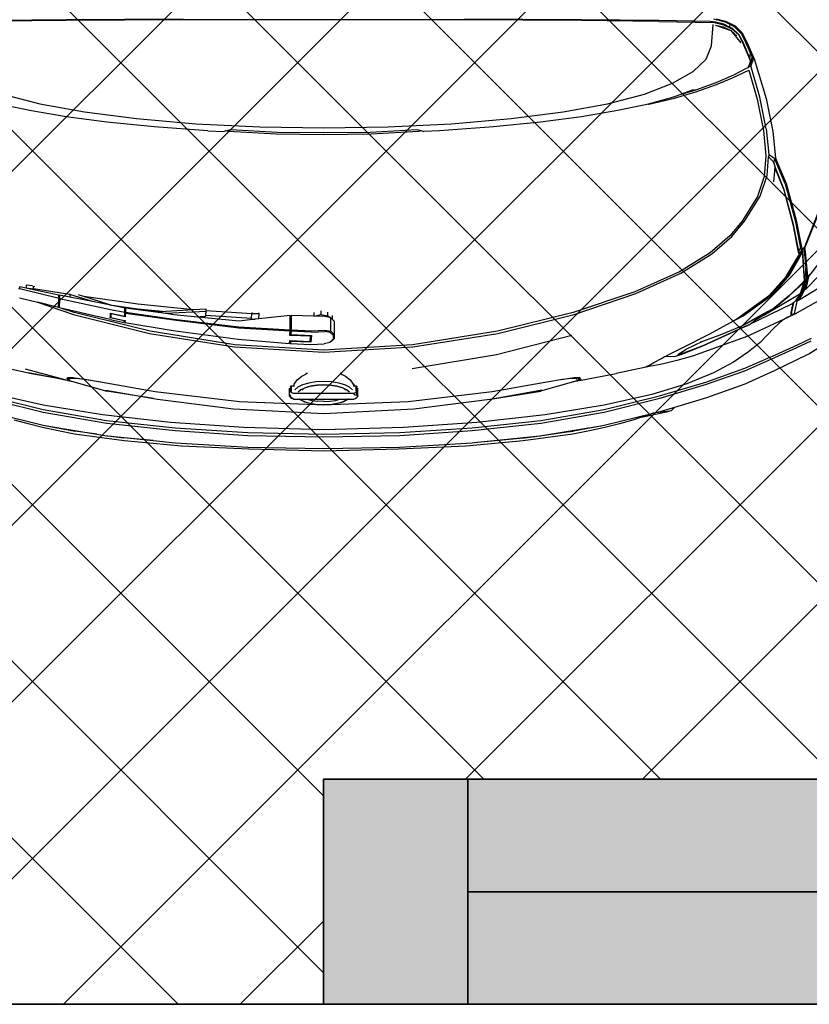
# Model space of a CAD drawing. Units: inches. Extents: x 2167 to 2589, y 1680 to 2489.
# Tile 13 of 38: x 2358 to 2389, y 1688 to 1727. Entities that reach past the tile are written whole.
import ezdxf

# ---------------------------------------------------------------- set-up
doc = ezdxf.new("R2010")
doc.units = ezdxf.units.IN
doc.header["$MEASUREMENT"] = 0
doc.layers.get('0').update_dxf_attribs({"color": 250})
for name, color, linetype, lineweight in [('A-WALL-PATT', 250, 'Continuous', 13), ('C-PRKG-VEHS', 8, 'Continuous', 13), ('C-PROP', 7, 'Continuous', 35), ('L-PVMT-PATT', 252, 'Continuous', 13), ('walls', 7, 'Continuous', 35)]:
    doc.layers.add(name, color=color, linetype=linetype, lineweight=lineweight)
doc.layers.add('Edges', color=250, linetype='Continuous')

# ---------------------------------------------------------------- blocks, each defined once
blk = doc.blocks.new('Nissan Qashqai pl')
at = {"layer": 'Edges'}
for p, q in [((11.3915, 12.6453), (11.4381, 12.6002)), ((11.417, 12.6499), (11.4529, 12.5922)), ((11.4203, 12.6044), (11.3733, 12.6404)), ((11.4732, 12.585), (11.4462, 12.6324)), ((11.3751, 12.5999), (11.3311, 12.6172)), ((11.3747, 12.6011), (11.3323, 12.6178)), ((11.5295, 12.6041), (11.5158, 12.6256)), ((11.38, 12.5988), (11.3747, 12.6011)), ((11.4212, 12.603), (11.3853, 12.5993)), ((11.4152, 12.6004), (11.409, 12.5999)), ((11.4173, 12.6006), (11.4152, 12.6004)), ((11.4163, 12.5999), (11.4152, 12.6004)), ((11.4176, 12.6007), (11.4173, 12.6006)), ((11.418, 12.6006), (11.4173, 12.6006)), ((11.4215, 12.601), (11.4176, 12.6007)), ((11.418, 12.6006), (11.4176, 12.6007)), ((11.4177, 12.6052), (11.4193, 12.6042)), ((11.4204, 12.6002), (11.418, 12.6006)), ((11.4194, 12.6), (11.418, 12.6006)), ((11.4192, 12.6045), (11.4194, 12.6042)), ((11.4194, 12.6042), (11.4193, 12.6042)), ((11.4193, 12.6042), (11.4196, 12.604)), ((11.4194, 12.6042), (11.4196, 12.604)), ((11.4196, 12.6042), (11.4194, 12.6042)), ((11.4196, 12.604), (11.4201, 12.6036)), ((11.4198, 12.6041), (11.4201, 12.6036)), ((11.4201, 12.6036), (11.4212, 12.603)), ((11.4292, 12.6024), (11.4203, 12.6044)), ((11.4229, 12.6025), (11.4203, 12.6044)), ((11.4212, 12.603), (11.4215, 12.601)), ((11.4218, 12.6028), (11.4212, 12.603)), ((11.4215, 12.601), (11.4219, 12.6009)), ((11.4222, 12.6029), (11.4218, 12.6028)), ((11.4229, 12.6025), (11.4218, 12.6028)), ((11.4219, 12.6009), (11.4222, 12.6005)), ((11.4219, 12.6009), (11.4224, 12.6008)), ((11.4224, 12.6008), (11.4226, 12.6006)), ((11.4224, 12.6008), (11.423, 12.6006)), ((11.4315, 12.6002), (11.4229, 12.6025)), ((11.423, 12.6006), (11.4229, 12.6025)), ((11.44, 12.5959), (11.423, 12.6006)), ((11.4381, 12.6002), (11.4292, 12.6024)), ((11.5165, 12.5882), (11.5074, 12.608)), ((11.5113, 12.6068), (11.5206, 12.5869)), ((11.5384, 12.5859), (11.5295, 12.6041)), ((11.3411, 12.5863), (11.3795, 12.5939)), ((11.3419, 12.585), (11.3804, 12.5926)), ((11.3847, 12.5899), (11.3474, 12.5827)), ((11.3863, 12.5898), (11.3493, 12.5828)), ((11.3751, 12.5999), (11.3762, 12.5999)), ((11.3752, 12.5998), (11.3751, 12.5999)), ((11.3763, 12.5998), (11.3752, 12.5998)), ((11.3764, 12.5993), (11.3752, 12.5998)), ((11.3792, 12.5982), (11.3764, 12.5993)), ((11.3792, 12.5982), (11.3793, 12.5979)), ((11.3792, 12.5982), (11.3804, 12.5972)), ((11.3795, 12.5939), (11.3834, 12.5947)), ((11.3853, 12.5993), (11.38, 12.5988)), ((11.3804, 12.5972), (11.4082, 12.5998)), ((11.3827, 12.5953), (11.3804, 12.5972)), ((11.3804, 12.5926), (11.3841, 12.5933)), ((11.3847, 12.5899), (11.3804, 12.5926)), ((11.3811, 12.5958), (11.3808, 12.5961)), ((11.3834, 12.5947), (11.3827, 12.5953)), ((11.3846, 12.5953), (11.3829, 12.5952)), ((11.3829, 12.5952), (11.3849, 12.5951)), ((11.388, 12.591), (11.3829, 12.5952)), ((11.3834, 12.5947), (11.3841, 12.5933)), ((11.3846, 12.5953), (11.4248, 12.5976)), ((11.3846, 12.5953), (11.3846, 12.5953)), ((11.3851, 12.5951), (11.3846, 12.5953)), ((11.3846, 12.5953), (11.3849, 12.5951)), ((11.3847, 12.5899), (11.3848, 12.5899)), ((11.388, 12.591), (11.3848, 12.5899)), ((11.3849, 12.5951), (11.3851, 12.5951)), ((11.3882, 12.5923), (11.3849, 12.5951)), ((11.3851, 12.5951), (11.3867, 12.5949)), ((11.4171, 12.5766), (11.3851, 12.5951)), ((11.3895, 12.5912), (11.3863, 12.5898)), ((11.3867, 12.5949), (11.3915, 12.5951)), ((11.3914, 12.5926), (11.3867, 12.5949)), ((11.3886, 12.5919), (11.3872, 12.5927)), ((11.3882, 12.5923), (11.3886, 12.5919)), ((11.3886, 12.5919), (11.3895, 12.5912)), ((11.3892, 12.5916), (11.3886, 12.5919)), ((11.3923, 12.5894), (11.3895, 12.5912)), ((11.4187, 12.5768), (11.3914, 12.5926)), ((11.3915, 12.5951), (11.4266, 12.5977)), ((11.4203, 12.5724), (11.3923, 12.5894)), ((11.409, 12.5999), (11.4082, 12.5998)), ((11.4164, 12.5998), (11.4082, 12.5998)), ((11.409, 12.5999), (11.4163, 12.5999)), ((11.4163, 12.5999), (11.4186, 12.5999)), ((11.4164, 12.5998), (11.4163, 12.5999)), ((11.4181, 12.5998), (11.4164, 12.5998)), ((11.4169, 12.5996), (11.4164, 12.5998)), ((11.4252, 12.598), (11.4169, 12.5996)), ((11.4248, 12.5976), (11.4266, 12.5977)), ((11.4266, 12.5977), (11.4252, 12.598)), ((11.4266, 12.5977), (11.4268, 12.5977)), ((11.4268, 12.5977), (11.4296, 12.5954)), ((11.4268, 12.5977), (11.4278, 12.5977)), ((11.4303, 12.5956), (11.4278, 12.5977)), ((11.4278, 12.5977), (11.43, 12.5969)), ((11.4296, 12.5954), (11.4469, 12.5773)), ((11.4337, 12.5962), (11.43, 12.5969)), ((11.43, 12.5969), (11.4361, 12.5948)), ((11.4479, 12.5766), (11.4303, 12.5956)), ((11.4403, 12.5978), (11.4315, 12.6002)), ((11.4397, 12.5937), (11.4337, 12.5962)), ((11.4361, 12.5948), (11.4406, 12.5932)), ((11.4381, 12.6002), (11.4403, 12.5978)), ((11.4406, 12.5932), (11.4397, 12.5937)), ((11.4403, 12.5978), (11.44, 12.5959)), ((11.44, 12.5959), (11.4457, 12.5928)), ((11.4462, 12.5947), (11.4403, 12.5978)), ((11.4406, 12.5932), (11.4442, 12.592)), ((11.4442, 12.592), (11.4497, 12.589)), ((11.4462, 12.5893), (11.4442, 12.592)), ((11.4457, 12.5928), (11.4512, 12.5893)), ((11.452, 12.591), (11.4462, 12.5947)), ((11.475, 12.5409), (11.4462, 12.5893)), ((11.4497, 12.589), (11.4498, 12.5889)), ((11.4535, 12.5876), (11.4498, 12.5889)), ((11.4498, 12.5889), (11.4549, 12.5855)), ((11.4512, 12.5893), (11.4535, 12.5876)), ((11.4539, 12.5897), (11.452, 12.591)), ((11.4529, 12.5922), (11.4542, 12.5894)), ((11.4535, 12.5876), (11.4532, 12.5882)), ((11.4535, 12.5876), (11.4542, 12.5894)), ((11.4535, 12.5876), (11.4728, 12.5838)), ((11.4542, 12.5894), (11.4539, 12.5897)), ((11.5306, 12.5573), (11.5165, 12.5882)), ((11.5206, 12.5869), (11.5349, 12.5559)), ((11.2895, 12.5724), (11.3411, 12.5863)), ((11.29, 12.5711), (11.3419, 12.585)), ((11.3474, 12.5827), (11.2972, 12.5692)), ((11.3493, 12.5828), (11.2993, 12.5695)), ((11.3474, 12.5827), (11.3474, 12.5827)), ((11.4433, 12.5543), (11.4171, 12.5766)), ((11.4447, 12.5545), (11.4187, 12.5768)), ((11.4469, 12.5773), (11.4659, 12.5539)), ((11.4654, 12.5548), (11.4479, 12.5766)), ((11.4549, 12.5855), (11.4568, 12.5836)), ((11.4564, 12.5833), (11.4567, 12.5833)), ((11.4569, 12.583), (11.4565, 12.5831)), ((11.4568, 12.5836), (11.4571, 12.5833)), ((11.4571, 12.5833), (11.4573, 12.583)), ((11.4573, 12.583), (11.4578, 12.5822)), ((11.4704, 12.5803), (11.4573, 12.583)), ((11.4573, 12.5823), (11.4574, 12.5822)), ((11.4573, 12.5823), (11.4573, 12.5823)), ((11.4576, 12.5822), (11.4574, 12.5822)), ((11.4578, 12.5822), (11.4588, 12.5807)), ((11.4605, 12.5816), (11.4578, 12.5822)), ((11.4588, 12.5807), (11.4895, 12.5178)), ((11.4713, 12.5794), (11.4605, 12.5816)), ((11.4742, 12.5797), (11.4704, 12.5803)), ((11.4744, 12.5792), (11.4713, 12.5794)), ((11.4732, 12.585), (11.4728, 12.5838)), ((11.4728, 12.5838), (11.4742, 12.5797)), ((11.4728, 12.5838), (11.4746, 12.5796)), ((11.4758, 12.5791), (11.4732, 12.585)), ((11.4742, 12.5797), (11.4744, 12.5792)), ((11.4745, 12.5797), (11.4742, 12.5797)), ((11.4745, 12.5792), (11.4744, 12.5792)), ((11.4745, 12.5792), (11.4745, 12.5797)), ((11.4745, 12.5797), (11.4746, 12.5796)), ((11.4748, 12.5792), (11.4745, 12.5792)), ((11.4746, 12.5796), (11.4748, 12.5792)), ((11.4746, 12.5796), (11.4758, 12.5791)), ((11.4758, 12.5791), (11.4748, 12.5792)), ((11.4758, 12.5791), (11.4759, 12.579)), ((11.4759, 12.579), (11.4778, 12.5746)), ((11.4759, 12.579), (11.4771, 12.576)), ((11.5057, 12.5145), (11.4771, 12.576)), ((11.4778, 12.5746), (11.4826, 12.5669)), ((11.5527, 12.5559), (11.5384, 12.5859)), ((11.2538, 12.5571), (11.2586, 12.5591)), ((11.29, 12.5711), (11.2541, 12.5557)), ((11.2586, 12.5591), (11.2895, 12.5724)), ((11.2972, 12.5692), (11.2677, 12.5575)), ((11.2993, 12.5695), (11.2705, 12.5579)), ((11.4467, 12.5488), (11.4203, 12.5724)), ((11.4633, 12.5594), (11.4897, 12.5108)), ((11.4826, 12.5669), (11.4869, 12.5615)), ((11.4869, 12.5615), (11.4933, 12.555)), ((11.1702, 12.5444), (11.2166, 12.5534)), ((11.2127, 12.5443), (11.2488, 12.548)), ((11.2166, 12.5534), (11.2538, 12.5571)), ((11.2488, 12.548), (11.2541, 12.5557)), ((11.2488, 12.548), (11.2524, 12.5477)), ((11.2599, 12.5552), (11.2524, 12.5477)), ((11.2785, 12.5455), (11.2524, 12.5477)), ((11.2541, 12.5557), (11.2599, 12.5552)), ((11.2677, 12.5575), (11.2599, 12.5552)), ((11.265, 12.5563), (11.2599, 12.5552)), ((11.2705, 12.5579), (11.265, 12.5563)), ((11.265, 12.5563), (11.2724, 12.5557)), ((11.2724, 12.5557), (11.2874, 12.5544)), ((11.3076, 12.5358), (11.2785, 12.5455)), ((11.4745, 12.5116), (11.4433, 12.5543)), ((11.4758, 12.5118), (11.4447, 12.5545)), ((11.4801, 12.503), (11.4467, 12.5488)), ((11.4654, 12.5548), (11.4659, 12.5539)), ((11.4659, 12.5539), (11.4674, 12.5512)), ((11.4675, 12.551), (11.4674, 12.5512)), ((11.4675, 12.551), (11.4703, 12.546)), ((11.4703, 12.546), (11.4704, 12.5458)), ((11.4704, 12.5458), (11.4909, 12.5085)), ((11.4704, 12.5458), (11.4897, 12.5108)), ((11.5131, 12.5356), (11.4933, 12.555)), ((11.5496, 12.5141), (11.5306, 12.5573)), ((11.5349, 12.5559), (11.5535, 12.5139)), ((11.5716, 12.5145), (11.5527, 12.5559)), ((11.1144, 12.5271), (11.1702, 12.5444)), ((11.1683, 12.5354), (11.1244, 12.5227)), ((11.1302, 12.52), (11.1712, 12.5317)), ((11.2127, 12.5443), (11.1683, 12.5354)), ((11.1712, 12.5317), (11.2152, 12.5404)), ((11.2152, 12.5404), (11.2509, 12.5439)), ((11.2509, 12.5439), (11.28, 12.5414)), ((11.28, 12.5414), (11.3082, 12.532)), ((11.3428, 12.5139), (11.3076, 12.5358)), ((11.3082, 12.532), (11.3425, 12.5106)), ((11.475, 12.5409), (11.4828, 12.5276)), ((11.5131, 12.5356), (11.5265, 12.5194)), ((11.0902, 12.5166), (11.1144, 12.5271)), ((11.0908, 12.5153), (11.107, 12.5224)), ((11.1138, 12.5213), (11.0912, 12.5117)), ((11.1149, 12.5212), (11.0917, 12.5114)), ((11.107, 12.5224), (11.1116, 12.5243)), ((11.1138, 12.5213), (11.107, 12.5224)), ((11.1116, 12.5243), (11.1147, 12.5257)), ((11.1244, 12.5227), (11.1116, 12.5243)), ((11.1139, 12.5213), (11.1138, 12.5213)), ((11.1164, 12.5224), (11.1139, 12.5213)), ((11.1147, 12.5257), (11.1244, 12.5227)), ((11.1172, 12.5222), (11.1149, 12.5212)), ((11.1164, 12.5224), (11.1174, 12.5223)), ((11.1173, 12.5222), (11.1172, 12.5222)), ((11.1174, 12.5223), (11.1173, 12.5222)), ((11.12, 12.5215), (11.1174, 12.5223)), ((11.1246, 12.5199), (11.12, 12.5215)), ((11.1259, 12.5194), (11.1244, 12.5227)), ((11.1244, 12.5227), (11.126, 12.5194)), ((11.1259, 12.5194), (11.1246, 12.5199)), ((11.126, 12.5193), (11.1247, 12.5197)), ((11.126, 12.5193), (11.1248, 12.5195)), ((11.1251, 12.5189), (11.126, 12.5193)), ((11.126, 12.5193), (11.1259, 12.5194)), ((11.126, 12.5194), (11.1259, 12.5194)), ((11.126, 12.5194), (11.1261, 12.5193)), ((11.1264, 12.5192), (11.126, 12.5194)), ((11.1263, 12.5186), (11.126, 12.5193)), ((11.1261, 12.5193), (11.126, 12.5193)), ((11.1261, 12.5193), (11.1263, 12.5188)), ((11.1264, 12.5192), (11.1261, 12.5193)), ((11.1277, 12.5167), (11.1264, 12.5192)), ((11.1412, 12.4969), (11.1302, 12.52)), ((11.488, 12.5208), (11.4828, 12.5276)), ((11.5179, 12.4551), (11.488, 12.5208)), ((11.4898, 12.5172), (11.4895, 12.5178)), ((11.4898, 12.5172), (11.49, 12.5167)), ((11.5265, 12.5194), (11.541, 12.4982)), ((11.0682, 12.5004), (11.0779, 12.5103)), ((11.0692, 12.4996), (11.0787, 12.5092)), ((11.0802, 12.5057), (11.0718, 12.4967)), ((11.0809, 12.5056), (11.0727, 12.4966)), ((11.0747, 12.4944), (11.092, 12.5087)), ((11.0779, 12.5103), (11.0902, 12.5166)), ((11.0787, 12.5092), (11.0908, 12.5153)), ((11.0912, 12.5117), (11.0802, 12.5057)), ((11.0917, 12.5114), (11.0809, 12.5056)), ((11.1369, 12.4986), (11.1277, 12.5167)), ((11.3425, 12.5106), (11.3635, 12.4929)), ((11.3645, 12.4958), (11.3428, 12.5139)), ((11.4788, 12.5052), (11.4745, 12.5116)), ((11.4852, 12.494), (11.4758, 12.5118)), ((11.4801, 12.503), (11.4788, 12.5052)), ((11.4897, 12.5108), (11.4909, 12.5085)), ((11.49, 12.5167), (11.5179, 12.4551)), ((11.4909, 12.5085), (11.5028, 12.4792)), ((11.5057, 12.5145), (11.5325, 12.4404)), ((11.5691, 12.4592), (11.5496, 12.5141)), ((11.5535, 12.5139), (11.5726, 12.46)), ((11.5908, 12.4606), (11.5716, 12.5145)), ((11.0614, 12.4872), (11.0682, 12.5004)), ((11.0624, 12.4866), (11.0658, 12.4932)), ((11.0658, 12.4932), (11.0692, 12.4996)), ((11.0658, 12.4932), (11.0698, 12.4925)), ((11.0698, 12.4925), (11.0659, 12.4848)), ((11.0727, 12.4966), (11.0669, 12.4849)), ((11.0671, 12.4731), (11.0747, 12.4944)), ((11.0696, 12.4836), (11.0747, 12.4944)), ((11.0718, 12.4967), (11.0698, 12.4925)), ((11.0747, 12.4944), (11.0821, 12.5029)), ((11.1475, 12.4741), (11.1369, 12.4986)), ((11.1505, 12.4742), (11.1412, 12.4969)), ((11.3635, 12.4929), (11.3872, 12.4654)), ((11.3888, 12.4678), (11.3645, 12.4958)), ((11.4852, 12.494), (11.4801, 12.503)), ((11.5013, 12.4651), (11.4852, 12.494)), ((11.541, 12.4982), (11.5562, 12.4701)), ((11.0581, 12.4738), (11.0614, 12.4872)), ((11.0582, 12.47), (11.0624, 12.4866)), ((11.0659, 12.4848), (11.063, 12.4728)), ((11.0669, 12.4849), (11.0641, 12.4733)), ((11.0671, 12.4731), (11.0696, 12.4836)), ((11.5028, 12.4792), (11.5118, 12.4548)), ((11.0621, 12.4657), (11.0607, 12.3933)), ((11.0618, 12.3933), (11.0632, 12.47)), ((11.0622, 12.4697), (11.0621, 12.4657)), ((11.063, 12.4728), (11.0622, 12.4697)), ((11.0641, 12.4733), (11.0632, 12.47)), ((11.0962, 12.4675), (11.0662, 12.4698)), ((11.1148, 12.4598), (11.0962, 12.4675)), ((11.1577, 12.4465), (11.1475, 12.4741)), ((11.1605, 12.4465), (11.1505, 12.4742)), ((11.3872, 12.4654), (11.4138, 12.4223)), ((11.4159, 12.4242), (11.3888, 12.4678)), ((11.5202, 12.427), (11.5013, 12.4651)), ((11.5562, 12.4701), (11.5715, 12.4326)), ((11.1323, 12.4415), (11.1148, 12.4598)), ((11.5118, 12.4548), (11.523, 12.4311)), ((11.5118, 12.4548), (11.513, 12.4514)), ((11.5292, 12.4272), (11.5179, 12.4551)), ((11.5179, 12.4551), (11.5285, 12.4279)), ((11.5884, 12.3943), (11.5691, 12.4592)), ((11.5726, 12.46), (11.5922, 12.3947)), ((11.6042, 12.4156), (11.5908, 12.4606)), ((11.1487, 12.4126), (11.1323, 12.4415)), ((11.1643, 12.425), (11.1576, 12.4459)), ((11.1643, 12.425), (11.1577, 12.4465)), ((11.1582, 12.4416), (11.1668, 12.4177)), ((11.1583, 12.4423), (11.1643, 12.425)), ((11.1699, 12.4153), (11.1605, 12.4465)), ((11.5325, 12.4404), (11.5386, 12.4187)), ((11.1643, 12.425), (11.1668, 12.4177)), ((11.4138, 12.4223), (11.4422, 12.3594)), ((11.4445, 12.3608), (11.4159, 12.4242)), ((11.5283, 12.4109), (11.5202, 12.427)), ((11.5301, 12.4198), (11.523, 12.4311)), ((11.5285, 12.4279), (11.5302, 12.4209)), ((11.5331, 12.4157), (11.5292, 12.4272)), ((11.5302, 12.4209), (11.5301, 12.4198)), ((11.5715, 12.4326), (11.5866, 12.3835)), ((11.164, 12.373), (11.1487, 12.4126)), ((11.1668, 12.4177), (11.1694, 12.4104)), ((11.1694, 12.4104), (11.1781, 12.3782)), ((11.178, 12.379), (11.1699, 12.4153)), ((11.5334, 12.4014), (11.5283, 12.4109)), ((11.5331, 12.4157), (11.5335, 12.401)), ((11.5386, 12.4187), (11.5434, 12.3997)), ((11.6042, 12.4156), (11.6077, 12.4125)), ((11.6103, 12.395), (11.6042, 12.4156)), ((11.6077, 12.4125), (11.6094, 12.4107)), ((11.6094, 12.4107), (11.6101, 12.4085)), ((11.6101, 12.4085), (11.6127, 12.3852)), ((11.6185, 12.3689), (11.6101, 12.4085)), ((11.0607, 12.3933), (11.0595, 12.2842)), ((11.0618, 12.3933), (11.0606, 12.2841)), ((11.5326, 12.4045), (11.5333, 12.4019)), ((11.5333, 12.4019), (11.5334, 12.4014)), ((11.5335, 12.401), (11.5334, 12.4014)), ((11.5357, 12.3968), (11.5335, 12.401)), ((11.5416, 12.3863), (11.5357, 12.3968)), ((11.5434, 12.3997), (11.5461, 12.3854)), ((11.6076, 12.3166), (11.5884, 12.3943)), ((11.5922, 12.3947), (11.6118, 12.3165)), ((11.6127, 12.3852), (11.6103, 12.395)), ((11.1781, 12.3782), (11.178, 12.379)), ((11.5455, 12.3793), (11.5416, 12.3863)), ((11.5472, 12.3757), (11.5455, 12.3793)), ((11.5461, 12.3854), (11.5467, 12.3822)), ((11.5467, 12.3822), (11.5571, 12.3331)), ((11.5866, 12.3835), (11.6016, 12.3166)), ((11.6127, 12.3852), (11.6174, 12.3722)), ((11.6297, 12.3166), (11.6127, 12.3852)), ((11.1776, 12.3211), (11.164, 12.373)), ((11.1781, 12.3782), (11.1791, 12.3746)), ((11.1791, 12.3746), (11.1877, 12.333)), ((11.6174, 12.3722), (11.6185, 12.3689)), ((11.6185, 12.3689), (11.6224, 12.3567)), ((11.4422, 12.3594), (11.4712, 12.2729)), ((11.4738, 12.274), (11.4445, 12.3608)), ((11.6224, 12.3567), (11.6277, 12.3379)), ((11.6277, 12.3379), (11.6328, 12.3174)), ((11.1877, 12.333), (11.1958, 12.2844)), ((11.5668, 12.2816), (11.5571, 12.3331)), ((11.1891, 12.2586), (11.1776, 12.3211)), ((11.6016, 12.3166), (11.615, 12.2333)), ((11.6229, 12.2274), (11.6076, 12.3166)), ((11.6118, 12.3165), (11.6272, 12.2272)), ((11.6301, 12.3141), (11.6297, 12.3166)), ((11.6377, 12.2734), (11.6301, 12.3141)), ((11.6332, 12.2951), (11.6301, 12.3141)), ((11.6328, 12.3174), (11.6375, 12.2956)), ((11.0595, 12.2842), (11.0586, 12.1198)), ((11.0606, 12.2841), (11.0597, 12.1196)), ((11.1958, 12.2844), (11.2033, 12.2269)), ((11.5627, 12.2817), (11.5634, 12.2829)), ((11.5633, 12.2814), (11.5634, 12.2829)), ((11.5634, 12.2829), (11.5668, 12.2816)), ((11.566, 12.2846), (11.5668, 12.2816)), ((11.6334, 12.2946), (11.6332, 12.2951)), ((11.6443, 12.2288), (11.6334, 12.2946)), ((11.6375, 12.2956), (11.6422, 12.2725)), ((11.4712, 12.2729), (11.4976, 12.1662)), ((11.5005, 12.167), (11.4738, 12.274)), ((11.5033, 12.271), (11.5307, 12.165)), ((11.5626, 12.2771), (11.5627, 12.2817)), ((11.5627, 12.2746), (11.5626, 12.2771)), ((11.5626, 12.2745), (11.5627, 12.2746)), ((11.5627, 12.2817), (11.5633, 12.2814)), ((11.5628, 12.2721), (11.5627, 12.2746)), ((11.5632, 12.2783), (11.5633, 12.2814)), ((11.5636, 12.2706), (11.5632, 12.2783)), ((11.5633, 12.2814), (11.5661, 12.2803)), ((11.565, 12.2577), (11.5636, 12.2706)), ((11.5639, 12.2809), (11.5637, 12.2764)), ((11.5637, 12.2763), (11.5637, 12.2764)), ((11.5637, 12.2764), (11.5638, 12.2762)), ((11.5638, 12.2762), (11.5641, 12.2688)), ((11.5643, 12.2808), (11.5639, 12.2809)), ((11.5641, 12.2688), (11.5656, 12.2559)), ((11.5642, 12.2771), (11.5646, 12.2778)), ((11.566, 12.2801), (11.5643, 12.2808)), ((11.5647, 12.278), (11.5649, 12.2783)), ((11.566, 12.2801), (11.5661, 12.2803)), ((11.5662, 12.28), (11.566, 12.2801)), ((11.5661, 12.2803), (11.5662, 12.28)), ((11.5662, 12.28), (11.5661, 12.2803)), ((11.5669, 12.2797), (11.5661, 12.2803)), ((11.5669, 12.2797), (11.5662, 12.28)), ((11.5662, 12.28), (11.5662, 12.28)), ((11.5667, 12.2813), (11.567, 12.2796)), ((11.5668, 12.2816), (11.5672, 12.2796)), ((11.567, 12.2796), (11.5669, 12.2797)), ((11.5672, 12.2796), (11.567, 12.2796)), ((11.5678, 12.2766), (11.5672, 12.2796)), ((11.5673, 12.2784), (11.5677, 12.2767)), ((11.5678, 12.2766), (11.5818, 12.227)), ((11.5682, 12.2743), (11.5682, 12.2742)), ((11.5683, 12.2739), (11.5683, 12.2739)), ((11.5683, 12.2738), (11.5683, 12.2737)), ((11.6378, 12.2728), (11.6377, 12.2734)), ((11.6381, 12.2716), (11.6378, 12.2728)), ((11.639, 12.2645), (11.6378, 12.2728)), ((11.639, 12.2645), (11.6381, 12.2716)), ((11.6422, 12.2725), (11.6514, 12.2026)), ((11.1984, 12.1855), (11.1891, 12.2586)), ((11.5685, 12.2359), (11.565, 12.2577)), ((11.6443, 12.2288), (11.639, 12.2645)), ((11.2033, 12.2269), (11.21, 12.1607)), ((11.5823, 12.1589), (11.5685, 12.2359)), ((11.593, 12.1566), (11.58, 12.2288)), ((11.5883, 12.186), (11.5816, 12.2272)), ((11.5883, 12.186), (11.5818, 12.227)), ((11.615, 12.2333), (11.626, 12.1375)), ((11.6333, 12.131), (11.6229, 12.2274)), ((11.6272, 12.2272), (11.6377, 12.1308)), ((11.6446, 12.2271), (11.6443, 12.2288)), ((11.6448, 12.2258), (11.6446, 12.2271)), ((11.6474, 12.2042), (11.6448, 12.2258)), ((11.6539, 12.1338), (11.6448, 12.2258)), ((11.6474, 12.2038), (11.6474, 12.2042)), ((11.6475, 12.2032), (11.6474, 12.2038)), ((11.648, 12.198), (11.6475, 12.2032)), ((11.6514, 12.2026), (11.6589, 12.1222)), ((11.2057, 12.1019), (11.1984, 12.1855)), ((11.593, 12.1566), (11.5883, 12.186)), ((11.6539, 12.1338), (11.648, 12.198)), ((11.21, 12.1607), (11.2159, 12.085)), ((11.4976, 12.1662), (11.5166, 12.0471)), ((11.5196, 12.0475), (11.5005, 12.167)), ((11.5307, 12.165), (11.5504, 12.0466)), ((11.5963, 12.0406), (11.5823, 12.1589)), ((11.5932, 12.1556), (11.593, 12.1566)), ((11.6067, 12.0489), (11.5932, 12.1556)), ((11.626, 12.1375), (11.6329, 12.0344)), ((11.6399, 12.029), (11.6333, 12.131)), ((11.6377, 12.1308), (11.6444, 12.0289)), ((11.6543, 12.1306), (11.6539, 12.1338)), ((11.6604, 12.0287), (11.6543, 12.1306)), ((11.0597, 12.1196), (11.0594, 11.9221)), ((11.6589, 12.1222), (11.6635, 12.0274)), ((11.2101, 12.012), (11.2057, 12.1019)), ((11.2159, 12.085), (11.2166, 12.063)), ((11.2158, 12.0602), (11.2166, 12.063)), ((11.2139, 12.0528), (11.2158, 12.0599)), ((11.2174, 11.9874), (11.2139, 12.0528)), ((11.2158, 12.0602), (11.2168, 12.056)), ((11.2158, 12.0599), (11.2158, 12.0602)), ((11.2158, 12.0599), (11.2168, 12.056)), ((11.2168, 12.056), (11.2204, 11.989)), ((11.5166, 12.0471), (11.5239, 11.9221)), ((11.527, 11.9221), (11.5196, 12.0475)), ((11.6133, 11.9221), (11.6067, 12.0489)), ((11.6005, 11.9335), (11.5963, 12.0406)), ((11.6329, 12.0344), (11.6363, 11.9221)), ((11.6421, 11.9221), (11.6399, 12.029)), ((11.6444, 12.0289), (11.6465, 11.9221)), ((11.6623, 11.9221), (11.6604, 12.0287)), ((11.6635, 12.0274), (11.6663, 11.9221)), ((11.2116, 11.9221), (11.2101, 12.012)), ((11.218, 11.9221), (11.2174, 11.9874)), ((11.2204, 11.989), (11.2211, 11.9221)), ((11.5659, 11.9594), (11.572, 11.9635)), ((11.572, 11.9635), (11.5746, 11.964)), ((11.5726, 11.9653), (11.5726, 11.9656)), ((11.5731, 11.9653), (11.5731, 11.9657)), ((11.5748, 11.9684), (11.5746, 11.9677)), ((11.5824, 11.9677), (11.5746, 11.9677)), ((11.5746, 11.9677), (11.5746, 11.964)), ((11.5746, 11.964), (11.5746, 11.9638)), ((11.5762, 11.9694), (11.5748, 11.9684)), ((11.5748, 11.9684), (11.5826, 11.9684)), ((11.5885, 11.9701), (11.5776, 11.9701)), ((11.5826, 11.9684), (11.5838, 11.9678)), ((11.5867, 11.9695), (11.5838, 11.9678)), ((11.5838, 11.9678), (11.5851, 11.9645)), ((11.5868, 11.966), (11.5851, 11.9645)), ((11.5851, 11.9645), (11.5851, 11.8796)), ((11.5868, 11.966), (11.5867, 11.9695)), ((11.5896, 11.9695), (11.5867, 11.9695)), ((11.5885, 11.9701), (11.5896, 11.9695)), ((11.5915, 11.9678), (11.5896, 11.9695)), ((11.5915, 11.9678), (11.5904, 11.9684)), ((11.5929, 11.9645), (11.5915, 11.9678)), ((11.5929, 11.9569), (11.5929, 11.9645)), ((11.5582, 11.9481), (11.5608, 11.9528)), ((11.5608, 11.9528), (11.5659, 11.9594)), ((11.5729, 11.9518), (11.5703, 11.9431)), ((11.5761, 11.9585), (11.5729, 11.9518)), ((11.5799, 11.9626), (11.5761, 11.9585)), ((11.5769, 11.9489), (11.5799, 11.9549)), ((11.5788, 11.9517), (11.5771, 11.9483)), ((11.58, 11.9542), (11.5788, 11.9517)), ((11.5788, 11.9517), (11.58, 11.953)), ((11.5799, 11.9549), (11.5829, 11.9582)), ((11.5829, 11.9574), (11.58, 11.9542)), ((11.5929, 11.9569), (11.5941, 11.9549)), ((11.5929, 11.9566), (11.5929, 11.9569)), ((11.5932, 11.9559), (11.5929, 11.9566)), ((11.5929, 11.9563), (11.5929, 11.9566)), ((11.5929, 11.9563), (11.5932, 11.9559)), ((11.5929, 11.9555), (11.5929, 11.9563)), ((11.594, 11.9542), (11.5929, 11.9555)), ((11.5929, 11.9453), (11.5929, 11.9555)), ((11.5932, 11.9559), (11.5941, 11.9549)), ((11.5969, 11.9483), (11.594, 11.9542)), ((11.5941, 11.9549), (11.5971, 11.9489)), ((11.4835, 11.937), (11.4811, 11.9346)), ((11.4835, 11.937), (11.5022, 11.937)), ((11.4974, 11.9321), (11.5022, 11.937)), ((11.5035, 11.9359), (11.4991, 11.9313)), ((11.5022, 11.937), (11.5081, 11.9367)), ((11.5089, 11.9356), (11.5035, 11.9359)), ((11.5081, 11.9367), (11.5129, 11.9312)), ((11.5565, 11.9451), (11.5564, 11.9475)), ((11.5565, 11.9451), (11.5582, 11.9481)), ((11.5703, 11.9431), (11.5688, 11.933)), ((11.5732, 11.9319), (11.5747, 11.941)), ((11.5749, 11.9407), (11.5735, 11.9317)), ((11.5747, 11.941), (11.5769, 11.9489)), ((11.5771, 11.9483), (11.5749, 11.9407)), ((11.5929, 11.8989), (11.5929, 11.9453)), ((11.5948, 11.9386), (11.5929, 11.9453)), ((11.596, 11.9306), (11.5948, 11.9386)), ((11.5991, 11.9407), (11.5969, 11.9483)), ((11.5971, 11.9489), (11.5993, 11.941)), ((11.6005, 11.9317), (11.5991, 11.9407)), ((11.5993, 11.941), (11.6005, 11.9335)), ((11.0594, 11.9221), (11.0597, 11.7245)), ((11.2101, 11.8322), (11.2116, 11.9221)), ((11.2174, 11.8567), (11.218, 11.9221)), ((11.2211, 11.9221), (11.2204, 11.8551)), ((11.4758, 11.928), (11.4706, 11.928)), ((11.474, 11.918), (11.4758, 11.928)), ((11.4811, 11.9346), (11.4755, 11.9346)), ((11.4758, 11.928), (11.4784, 11.9312)), ((11.4766, 11.9237), (11.4762, 11.9091)), ((11.4784, 11.9312), (11.4766, 11.9237)), ((11.4786, 11.9321), (11.4784, 11.9312)), ((11.4811, 11.9346), (11.4786, 11.9321)), ((11.4974, 11.9321), (11.4786, 11.9321)), ((11.4962, 11.9237), (11.4974, 11.9321)), ((11.4969, 11.9049), (11.4962, 11.9237)), ((11.4991, 11.9313), (11.498, 11.9236)), ((11.4986, 11.9049), (11.498, 11.9236)), ((11.5089, 11.9356), (11.5132, 11.9305)), ((11.5132, 11.9305), (11.5129, 11.9312)), ((11.5132, 11.9305), (11.5154, 11.9227)), ((11.5161, 11.9039), (11.5154, 11.9227)), ((11.5239, 11.9221), (11.5166, 11.7971)), ((11.5196, 11.7967), (11.527, 11.9221)), ((11.5688, 11.933), (11.5682, 11.9221)), ((11.5682, 11.9221), (11.5688, 11.9112)), ((11.5728, 11.9221), (11.5732, 11.9319)), ((11.5732, 11.9123), (11.5728, 11.9221)), ((11.5735, 11.9317), (11.573, 11.9221)), ((11.573, 11.9221), (11.5735, 11.9125)), ((11.5964, 11.9221), (11.596, 11.9306)), ((11.5964, 11.9221), (11.596, 11.9135)), ((11.6005, 11.9335), (11.6008, 11.9319)), ((11.601, 11.9221), (11.6005, 11.9317)), ((11.6005, 11.9125), (11.601, 11.9221)), ((11.6008, 11.9319), (11.6012, 11.9221)), ((11.6012, 11.9221), (11.6008, 11.9123)), ((11.6067, 11.7952), (11.6133, 11.9221)), ((11.6363, 11.9221), (11.6329, 11.8098)), ((11.6399, 11.8152), (11.6421, 11.9221)), ((11.6465, 11.9221), (11.6444, 11.8153)), ((11.6604, 11.8154), (11.6623, 11.9221)), ((11.6663, 11.9221), (11.6635, 11.8168)), ((11.469, 11.918), (11.474, 11.918)), ((11.471, 11.9083), (11.4762, 11.9083)), ((11.4762, 11.9091), (11.474, 11.918)), ((11.4762, 11.9083), (11.4754, 11.8761)), ((11.4762, 11.9091), (11.4762, 11.9083)), ((11.5688, 11.9112), (11.5703, 11.9011)), ((11.5747, 11.9032), (11.5732, 11.9123)), ((11.5735, 11.9125), (11.5749, 11.9035)), ((11.5948, 11.9056), (11.596, 11.9135)), ((11.5963, 11.8036), (11.6005, 11.9107)), ((11.5991, 11.9035), (11.6005, 11.9125)), ((11.6005, 11.9107), (11.5993, 11.9032)), ((11.6008, 11.9123), (11.6005, 11.9107)), ((11.4957, 11.8762), (11.4969, 11.9049)), ((11.4986, 11.9049), (11.4974, 11.8761)), ((11.5022, 11.8759), (11.5035, 11.9047)), ((11.5046, 11.9034), (11.5034, 11.8751)), ((11.5035, 11.9047), (11.513, 11.9041)), ((11.5118, 11.903), (11.5046, 11.9034)), ((11.5106, 11.8751), (11.5118, 11.903)), ((11.513, 11.9041), (11.5118, 11.8754)), ((11.5148, 11.8751), (11.5161, 11.9039)), ((11.5564, 11.8967), (11.5565, 11.8991)), ((11.5582, 11.896), (11.5565, 11.8991)), ((11.5608, 11.8913), (11.5582, 11.896)), ((11.5703, 11.9011), (11.5729, 11.8924)), ((11.5769, 11.8953), (11.5747, 11.9032)), ((11.5749, 11.9035), (11.5771, 11.8958)), ((11.5799, 11.8893), (11.5769, 11.8953)), ((11.5771, 11.8958), (11.5788, 11.8925)), ((11.5929, 11.8989), (11.5948, 11.9056)), ((11.5929, 11.8887), (11.5929, 11.8989)), ((11.594, 11.8899), (11.5969, 11.8958)), ((11.5971, 11.8953), (11.5941, 11.8893)), ((11.5969, 11.8958), (11.5991, 11.9035)), ((11.5993, 11.9032), (11.5971, 11.8953)), ((11.5659, 11.8848), (11.5608, 11.8913)), ((11.572, 11.8807), (11.5659, 11.8848)), ((11.5726, 11.8806), (11.572, 11.8807)), ((11.5726, 11.8806), (11.5726, 11.8808)), ((11.5731, 11.8805), (11.5726, 11.8806)), ((11.5729, 11.8924), (11.5761, 11.8857)), ((11.5731, 11.8805), (11.5731, 11.8808)), ((11.5746, 11.8802), (11.5731, 11.8805)), ((11.5746, 11.881), (11.5746, 11.8802)), ((11.5761, 11.8857), (11.5799, 11.8815)), ((11.58, 11.8912), (11.5788, 11.8925)), ((11.5788, 11.8925), (11.58, 11.8899)), ((11.5829, 11.886), (11.5799, 11.8893)), ((11.58, 11.8899), (11.5829, 11.8867)), ((11.5929, 11.8887), (11.594, 11.8899)), ((11.5929, 11.8872), (11.5941, 11.8893)), ((11.5929, 11.8879), (11.5929, 11.8887)), ((11.5929, 11.8876), (11.5932, 11.8883)), ((11.5932, 11.8883), (11.5929, 11.8879)), ((11.5929, 11.8876), (11.5929, 11.8879)), ((11.5929, 11.8872), (11.5929, 11.8876)), ((11.5929, 11.8796), (11.5929, 11.8872)), ((11.5941, 11.8893), (11.5932, 11.8883)), ((11.4754, 11.8761), (11.4945, 11.8762)), ((11.4956, 11.875), (11.4754, 11.8749)), ((11.4754, 11.8749), (11.4801, 11.831)), ((11.4913, 11.8028), (11.4956, 11.875)), ((11.4973, 11.8749), (11.493, 11.8027)), ((11.4945, 11.875), (11.4945, 11.8762)), ((11.4945, 11.8762), (11.4957, 11.8762)), ((11.5034, 11.8751), (11.4945, 11.875)), ((11.4973, 11.8749), (11.4956, 11.875)), ((11.4957, 11.8762), (11.4974, 11.8761)), ((11.5034, 11.8746), (11.4973, 11.8749)), ((11.4974, 11.8761), (11.5022, 11.8759)), ((11.5034, 11.8751), (11.5034, 11.8746)), ((11.5088, 11.8018), (11.5148, 11.8739)), ((11.5105, 11.8742), (11.5106, 11.8751)), ((11.5148, 11.8739), (11.5105, 11.8742)), ((11.5147, 11.8751), (11.5106, 11.8751)), ((11.5118, 11.8754), (11.5147, 11.8752)), ((11.5147, 11.8752), (11.5147, 11.8751)), ((11.5147, 11.8752), (11.5148, 11.8751)), ((11.5148, 11.8751), (11.5147, 11.8751)), ((11.5746, 11.8802), (11.5746, 11.8765)), ((11.5746, 11.8765), (11.5824, 11.8765)), ((11.5746, 11.8765), (11.5748, 11.8757)), ((11.5826, 11.8757), (11.5748, 11.8757)), ((11.5748, 11.8757), (11.5762, 11.8748)), ((11.5885, 11.8741), (11.5776, 11.8741)), ((11.5838, 11.8763), (11.5826, 11.8757)), ((11.5851, 11.8796), (11.5838, 11.8763)), ((11.5867, 11.8747), (11.5896, 11.8747)), ((11.5896, 11.8747), (11.5885, 11.8741)), ((11.5896, 11.8747), (11.5915, 11.8763)), ((11.5904, 11.8758), (11.5896, 11.8747)), ((11.5922, 11.8781), (11.5904, 11.8758)), ((11.5904, 11.8758), (11.5915, 11.8763)), ((11.5915, 11.8763), (11.5922, 11.8781)), ((11.5929, 11.8796), (11.5922, 11.8781)), ((11.2139, 11.7914), (11.2174, 11.8567)), ((11.2204, 11.8551), (11.2168, 11.7882)), ((11.2057, 11.7423), (11.2101, 11.8322)), ((11.473, 11.8314), (11.4716, 11.8314)), ((11.4801, 11.831), (11.473, 11.8314)), ((11.473, 11.8314), (11.473, 11.8209)), ((11.4801, 11.831), (11.4806, 11.8258)), ((11.4806, 11.8204), (11.4806, 11.8258)), ((11.4806, 11.8258), (11.4831, 11.803)), ((11.4728, 11.8209), (11.4687, 11.7567)), ((11.4711, 11.8209), (11.4719, 11.8209)), ((11.4728, 11.8209), (11.4719, 11.8209)), ((11.473, 11.8209), (11.4728, 11.8209)), ((11.4792, 11.8205), (11.473, 11.8209)), ((11.4751, 11.7564), (11.4792, 11.8205)), ((11.4806, 11.8204), (11.4792, 11.8205)), ((11.4792, 11.8205), (11.4792, 11.8205)), ((11.6333, 11.7132), (11.6399, 11.8152)), ((11.6444, 11.8153), (11.6377, 11.7134)), ((11.6543, 11.7136), (11.6604, 11.8154)), ((11.6635, 11.8168), (11.6589, 11.7219)), ((11.4831, 11.803), (11.4771, 11.7404)), ((11.4805, 11.7113), (11.4913, 11.8028)), ((11.493, 11.8027), (11.4821, 11.7112)), ((11.4964, 11.7104), (11.5088, 11.8018)), ((11.5823, 11.6852), (11.5963, 11.8036)), ((11.6329, 11.8098), (11.626, 11.7067)), ((11.2158, 11.7842), (11.2139, 11.7914)), ((11.2168, 11.7882), (11.2158, 11.784)), ((11.2168, 11.7882), (11.2158, 11.7842)), ((11.2158, 11.784), (11.2158, 11.7842)), ((11.2166, 11.7812), (11.2158, 11.784)), ((11.5166, 11.7971), (11.4976, 11.678)), ((11.5005, 11.6772), (11.5196, 11.7967)), ((11.5932, 11.6885), (11.6067, 11.7952)), ((11.2159, 11.7591), (11.2166, 11.7812)), ((11.2159, 11.7591), (11.21, 11.6835)), ((11.4687, 11.7567), (11.4665, 11.7568)), ((11.4665, 11.7568), (11.4676, 11.7389)), ((11.4698, 11.7567), (11.4687, 11.7567)), ((11.4698, 11.7567), (11.4727, 11.6999)), ((11.4751, 11.7564), (11.4698, 11.7567)), ((11.4761, 11.7564), (11.4751, 11.7564)), ((11.4771, 11.7404), (11.4761, 11.7564)), ((11.1984, 11.6587), (11.2057, 11.7423)), ((11.4676, 11.7389), (11.4594, 11.6607)), ((11.4676, 11.7389), (11.4699, 11.7001)), ((11.4771, 11.7404), (11.4743, 11.7114)), ((11.0586, 11.7244), (11.0595, 11.5599)), ((11.0597, 11.7245), (11.0606, 11.5601)), ((11.6589, 11.7219), (11.6514, 11.6415)), ((11.4709, 11.6433), (11.4805, 11.7113)), ((11.4821, 11.7112), (11.4726, 11.6432)), ((11.4743, 11.7114), (11.4727, 11.6999)), ((11.4854, 11.6425), (11.4964, 11.7104)), ((11.626, 11.7067), (11.615, 11.6108)), ((11.6229, 11.6168), (11.6333, 11.7132)), ((11.6377, 11.7134), (11.6272, 11.6169)), ((11.6511, 11.6823), (11.6543, 11.7136)), ((11.4705, 11.6909), (11.4642, 11.6385)), ((11.4727, 11.6999), (11.4651, 11.6434)), ((11.4658, 11.6603), (11.4699, 11.7001)), ((11.4699, 11.7001), (11.4705, 11.6909)), ((11.5922, 11.6828), (11.5932, 11.6885)), ((11.21, 11.6835), (11.2033, 11.6172)), ((11.4976, 11.678), (11.4712, 11.5713)), ((11.4738, 11.5702), (11.5005, 11.6772)), ((11.5685, 11.6083), (11.5823, 11.6852)), ((11.5802, 11.6156), (11.5922, 11.6828)), ((11.5922, 11.6828), (11.5818, 11.6172)), ((11.6448, 11.6184), (11.6511, 11.6823)), ((11.6511, 11.6823), (11.6475, 11.6409)), ((11.4594, 11.6607), (11.4487, 11.5846)), ((11.4602, 11.6212), (11.4658, 11.6603)), ((11.1891, 11.5856), (11.1984, 11.6587)), ((11.4642, 11.6385), (11.4611, 11.6241)), ((11.4651, 11.6426), (11.4642, 11.6385)), ((11.4651, 11.6434), (11.468, 11.6433)), ((11.4679, 11.6425), (11.4651, 11.6426)), ((11.4669, 11.6225), (11.4709, 11.6424)), ((11.468, 11.6433), (11.4679, 11.6425)), ((11.4709, 11.6424), (11.4679, 11.6425)), ((11.468, 11.6433), (11.4709, 11.6433)), ((11.4709, 11.6433), (11.4726, 11.6432)), ((11.4725, 11.6423), (11.4709, 11.6424)), ((11.4721, 11.6222), (11.4763, 11.6421)), ((11.4744, 11.6422), (11.4725, 11.6423)), ((11.4726, 11.6432), (11.4745, 11.6431)), ((11.4773, 11.643), (11.4731, 11.6231)), ((11.4744, 11.6422), (11.4745, 11.6431)), ((11.4763, 11.6421), (11.4744, 11.6422)), ((11.4745, 11.6431), (11.4773, 11.643)), ((11.4783, 11.6228), (11.4823, 11.6417)), ((11.483, 11.6417), (11.4788, 11.6219)), ((11.481, 11.6217), (11.4853, 11.6416)), ((11.4823, 11.6417), (11.4824, 11.6425)), ((11.4823, 11.6417), (11.483, 11.6417)), ((11.4824, 11.6425), (11.4825, 11.6427)), ((11.4853, 11.6425), (11.4824, 11.6425)), ((11.4825, 11.6427), (11.4853, 11.6425)), ((11.4853, 11.6416), (11.483, 11.6418)), ((11.483, 11.6418), (11.483, 11.6417)), ((11.4854, 11.6425), (11.4853, 11.6425)), ((11.6514, 11.6415), (11.6422, 11.5716)), ((11.6448, 11.6184), (11.6475, 11.6409)), ((11.2033, 11.6172), (11.1958, 11.5598)), ((11.4602, 11.6212), (11.4487, 11.5846)), ((11.4513, 11.5507), (11.4669, 11.6225)), ((11.4608, 11.6226), (11.4558, 11.5969)), ((11.4611, 11.6241), (11.4602, 11.6212)), ((11.4611, 11.6241), (11.4608, 11.6226)), ((11.481, 11.6217), (11.4649, 11.5526)), ((11.4749, 11.6221), (11.4721, 11.6222)), ((11.4731, 11.6231), (11.4751, 11.6229)), ((11.4749, 11.6221), (11.4751, 11.6229)), ((11.4788, 11.6219), (11.4749, 11.6221)), ((11.4751, 11.6229), (11.4783, 11.6228)), ((11.6446, 11.6171), (11.6448, 11.6184)), ((11.565, 11.5864), (11.5685, 11.6083)), ((11.5691, 11.6089), (11.5656, 11.5882)), ((11.5678, 11.5675), (11.5818, 11.6172)), ((11.615, 11.6108), (11.6016, 11.5276)), ((11.6076, 11.5276), (11.6229, 11.6168)), ((11.6272, 11.6169), (11.6118, 11.5276)), ((11.6423, 11.603), (11.6446, 11.6171)), ((11.4558, 11.5969), (11.4458, 11.5652)), ((11.4558, 11.5969), (11.4496, 11.5649)), ((11.6301, 11.53), (11.6423, 11.603)), ((11.6423, 11.603), (11.6381, 11.5726)), ((11.1776, 11.5231), (11.1891, 11.5856)), ((11.4472, 11.5801), (11.4464, 11.5774)), ((11.4487, 11.5846), (11.4472, 11.5801)), ((11.5636, 11.5736), (11.565, 11.5864)), ((11.5656, 11.5882), (11.5641, 11.5754)), ((11.4458, 11.5652), (11.438, 11.514)), ((11.4448, 11.5652), (11.4458, 11.5652)), ((11.4458, 11.5652), (11.4496, 11.5649)), ((11.4458, 11.5652), (11.4458, 11.5652)), ((11.4496, 11.5649), (11.4468, 11.5505)), ((11.4568, 11.5197), (11.4738, 11.5702)), ((11.4712, 11.5713), (11.4649, 11.5526)), ((11.5627, 11.5696), (11.5626, 11.5697)), ((11.5626, 11.567), (11.5627, 11.5696)), ((11.5627, 11.5624), (11.5626, 11.567)), ((11.5627, 11.5696), (11.5628, 11.5721)), ((11.5634, 11.5684), (11.5627, 11.5696)), ((11.5633, 11.5627), (11.5627, 11.5624)), ((11.5634, 11.5613), (11.5627, 11.5624)), ((11.5632, 11.5659), (11.5634, 11.5684)), ((11.5633, 11.5627), (11.5632, 11.5659)), ((11.5661, 11.5639), (11.5633, 11.5627)), ((11.5634, 11.5613), (11.5633, 11.5627)), ((11.5634, 11.5684), (11.5636, 11.5736)), ((11.5637, 11.5679), (11.5634, 11.5684)), ((11.5658, 11.5622), (11.5634, 11.5613)), ((11.5641, 11.5754), (11.5638, 11.5679)), ((11.5638, 11.5679), (11.5639, 11.5632)), ((11.5639, 11.5632), (11.5643, 11.5634)), ((11.5643, 11.5634), (11.566, 11.5641)), ((11.5649, 11.5659), (11.5647, 11.5662)), ((11.5661, 11.5639), (11.5658, 11.5622)), ((11.5662, 11.5624), (11.5658, 11.5622)), ((11.566, 11.5641), (11.5662, 11.5642)), ((11.5661, 11.5639), (11.566, 11.5641)), ((11.5662, 11.5642), (11.5661, 11.5639)), ((11.5661, 11.5639), (11.5662, 11.5642)), ((11.5661, 11.5639), (11.5665, 11.5641)), ((11.5661, 11.5639), (11.5661, 11.5639)), ((11.5662, 11.5642), (11.5665, 11.5643)), ((11.5667, 11.5642), (11.5662, 11.5624)), ((11.5662, 11.5642), (11.5662, 11.5642)), ((11.5662, 11.5624), (11.5665, 11.5641)), ((11.5666, 11.5625), (11.5662, 11.5624)), ((11.5665, 11.5643), (11.5667, 11.5644)), ((11.5665, 11.5641), (11.5665, 11.5643)), ((11.5665, 11.5641), (11.5667, 11.5642)), ((11.5668, 11.5626), (11.5665, 11.5614)), ((11.5666, 11.5625), (11.567, 11.5645)), ((11.5667, 11.5626), (11.5666, 11.5625)), ((11.5667, 11.5626), (11.5671, 11.5646)), ((11.5667, 11.5644), (11.5669, 11.5645)), ((11.5667, 11.5642), (11.5669, 11.5645)), ((11.5667, 11.5644), (11.5667, 11.5642)), ((11.5668, 11.5626), (11.5667, 11.5626)), ((11.5672, 11.5646), (11.5668, 11.5626)), ((11.5669, 11.5645), (11.567, 11.5645)), ((11.567, 11.5645), (11.5674, 11.5662)), ((11.567, 11.5645), (11.5671, 11.5646)), ((11.5671, 11.5646), (11.5676, 11.5671)), ((11.5671, 11.5646), (11.5672, 11.5646)), ((11.5672, 11.5646), (11.5676, 11.5671)), ((11.5675, 11.5665), (11.5674, 11.5662)), ((11.5676, 11.5671), (11.5678, 11.5675)), ((11.6301, 11.53), (11.6381, 11.5726)), ((11.6422, 11.5716), (11.6375, 11.5486)), ((11.0595, 11.5599), (11.0607, 11.4508)), ((11.0606, 11.5601), (11.0618, 11.4509)), ((11.1958, 11.5598), (11.1877, 11.5111)), ((11.4375, 11.4946), (11.4512, 11.5499)), ((11.4468, 11.5496), (11.4391, 11.5139)), ((11.4468, 11.5505), (11.45, 11.5507)), ((11.4498, 11.5498), (11.4468, 11.5496)), ((11.4498, 11.5498), (11.45, 11.5507)), ((11.4512, 11.5499), (11.4498, 11.5498)), ((11.45, 11.5507), (11.4513, 11.5507)), ((11.4529, 11.5498), (11.4512, 11.5499)), ((11.4513, 11.5507), (11.4529, 11.5507)), ((11.4529, 11.5507), (11.4571, 11.5505)), ((11.4571, 11.5496), (11.4529, 11.5498)), ((11.4643, 11.5491), (11.4568, 11.5197)), ((11.4571, 11.5505), (11.4599, 11.5503)), ((11.462, 11.5493), (11.4571, 11.5496)), ((11.4598, 11.5498), (11.4599, 11.5503)), ((11.464, 11.55), (11.4598, 11.5498)), ((11.4599, 11.5503), (11.462, 11.5502)), ((11.462, 11.5502), (11.464, 11.55)), ((11.4638, 11.5492), (11.462, 11.5493)), ((11.464, 11.55), (11.4638, 11.5492)), ((11.4643, 11.5491), (11.4638, 11.5492)), ((11.464, 11.55), (11.464, 11.55)), ((11.4642, 11.55), (11.464, 11.55)), ((11.464, 11.55), (11.4642, 11.55)), ((11.4642, 11.55), (11.4642, 11.55)), ((11.4643, 11.55), (11.4642, 11.55)), ((11.4649, 11.5526), (11.4643, 11.55)), ((11.5505, 11.5023), (11.5665, 11.5614)), ((11.5627, 11.5431), (11.5665, 11.5614)), ((11.6375, 11.5486), (11.6328, 11.5267)), ((11.5553, 11.5068), (11.5627, 11.5431)), ((11.5571, 11.511), (11.5627, 11.5431)), ((11.164, 11.4711), (11.1776, 11.5231)), ((11.6016, 11.5276), (11.5866, 11.4607)), ((11.5884, 11.4499), (11.6076, 11.5276)), ((11.6118, 11.5276), (11.5922, 11.4494)), ((11.6127, 11.4589), (11.6297, 11.5276)), ((11.6328, 11.5267), (11.6277, 11.5063)), ((11.6297, 11.5276), (11.6301, 11.53)), ((11.1877, 11.5111), (11.1791, 11.4696)), ((11.4337, 11.5124), (11.4325, 11.5038)), ((11.4347, 11.5141), (11.434, 11.5141)), ((11.435, 11.5158), (11.4347, 11.5141)), ((11.438, 11.514), (11.4347, 11.5141)), ((11.4382, 11.514), (11.4368, 11.5036)), ((11.4391, 11.5139), (11.4369, 11.5036)), ((11.4382, 11.514), (11.438, 11.514)), ((11.4391, 11.5139), (11.4382, 11.514)), ((11.4503, 11.4945), (11.4568, 11.5197)), ((11.5481, 11.471), (11.5571, 11.511)), ((11.4325, 11.5038), (11.4368, 11.5036)), ((11.4325, 11.5038), (11.4369, 11.5035)), ((11.4369, 11.5035), (11.435, 11.4947)), ((11.435, 11.4947), (11.439, 11.4927)), ((11.4375, 11.4946), (11.435, 11.4947)), ((11.4368, 11.5036), (11.4369, 11.5036)), ((11.4369, 11.5036), (11.4369, 11.5035)), ((11.6277, 11.5063), (11.6224, 11.4874))]:
    blk.add_line(p, q, dxfattribs=at)
blk = doc.blocks.new('car')
blk.add_blockref('Nissan Qashqai pl', (-9.7433, -11.9151))
blk = doc.blocks.new('carr')
blk.add_blockref('car', (0.5124, -0.007))

msp = doc.modelspace()

# ---------------------------------------------------------------- hatches: boundary and pattern name
at = {"layer": 'A-WALL-PATT'}
h = msp.add_hatch(color=256, dxfattribs=at)
h.dxf.hatch_style = 1
h.paths.add_polyline_path([(2575.048, 2029.695), (2422.048, 2029.695), (2422.048, 2161.695), (2427.018, 2161.695), (2427.018, 2161.941), (2427.018, 2166.195), (2417.548, 2166.195), (2417.548, 2025.195), (2575.048, 2025.195)])
h.paths.add_polyline_path([(2575.048, 2166.195), (2503.006, 2166.195), (2503.006, 2161.695), (2575.048, 2161.695)], flags=17)
h.paths.add_polyline_path([(2575.048, 2161.695), (2566.048, 2161.695), (2566.048, 2029.695), (2575.048, 2029.695)], flags=17)
h.paths.add_polyline_path([(2575.048, 2025.195), (2566.048, 2025.195), (2566.048, 1869.195), (2575.048, 1869.195)])
h.paths.add_polyline_path([(2575.048, 1869.195), (2566.048, 1869.195), (2447.7, 1869.195, -0.014764), (2447.737, 1867.924), (2447.737, 1864.695), (2575.048, 1864.695)])
h.paths.add_polyline_path([(2530.048, 1864.695), (2525.548, 1864.695), (2525.548, 1816.695), (2452.048, 1816.695), (2452.048, 1812.195), (2530.048, 1812.195)])
h.paths.add_polyline_path([(2455.041, 1830.653), (2452.048, 1830.653), (2452.048, 1816.695), (2455.041, 1816.695)], flags=17)
h.paths.add_polyline_path([(2575.048, 1864.695), (2566.048, 1864.695), (2566.048, 1788.195), (2456.097, 1788.195), (2456.097, 1783.941, -0.042065), (2455.697, 1779.195), (2527.685, 1779.195), (2527.685, 1687.695), (2532.185, 1687.695), (2532.185, 1779.195), (2575.048, 1779.195)])
h.paths.add_polyline_path([(2421.872, 1696.695), (2416.107, 1696.695), (2416.107, 1687.695), (2421.872, 1687.695)])
h.paths.add_polyline_path([(2375.607, 1696.695), (2369.843, 1696.695), (2369.843, 1687.695), (2375.607, 1687.695)])
h.paths.add_polyline_path([(2425.048, 2245.695), (2420.548, 2245.695), (2420.548, 2226.195), (2432.286, 2226.195), (2432.286, 2229.424), (2432.286, 2230.695), (2425.048, 2230.695)])
h.paths.add_polyline_path([(2224.048, 2151.195), (2318.548, 2151.195), (2318.548, 2177.304), (2314.783, 2177.304, -0.007324), (2314.048, 2177.315), (2314.048, 2155.695), (2224.048, 2155.695), (2224.048, 2157.455), (2215.048, 2157.455), (2215.048, 2103.585), (2218.974, 2103.585), (2224.048, 2103.585)])
at = {"layer": 'L-PVMT-PATT'}
h = msp.add_hatch(dxfattribs=at)
h.set_pattern_fill('ANSI37', color=256, scale=40)
h.paths.add_polyline_path([(2417.548, 1783.695), (2417.548, 1846.042), (2239.361, 1846.042), (2239.361, 1687.695), (2369.843, 1687.695), (2369.843, 1696.695), (2375.607, 1696.695), (2416.107, 1696.695), (2417.548, 1696.695)])
h = msp.add_hatch(color=256, dxfattribs=at)
h.dxf.hatch_style = 1
h.paths.add_polyline_path([(2416.107, 1696.695), (2375.607, 1696.695), (2375.607, 1692.195), (2416.107, 1692.195)])
h.paths.add_polyline_path([(2416.107, 1692.195), (2375.607, 1692.195), (2375.607, 1687.695), (2416.107, 1687.695)])

# ---------------------------------------------------------------- linework, layer by layer
at = {"layer": 'C-PROP'}
msp.add_line((2575.048, 1687.695), (2215.048, 1687.695), dxfattribs=at)
at = {"layer": 'walls'}
for p, q in [((2375.607, 1696.695), (2369.843, 1696.695)), ((2369.843, 1696.695), (2369.843, 1687.695)), ((2416.107, 1696.695), (2375.607, 1696.695)), ((2375.607, 1696.695), (2375.607, 1687.695)), ((2375.607, 1696.695), (2375.607, 1687.695)), ((2375.607, 1692.195), (2416.107, 1692.195))]:
    msp.add_line(p, q, dxfattribs=at)

# ---------------------------------------------------------------- block references
at = {"layer": 'C-PRKG-VEHS', "xscale": 28.42784210623918, "yscale": 28.42784210623918, "zscale": 28.42784210623918, "rotation": 270}
msp.add_blockref('carr', (2369.852, 1779.037), dxfattribs=at)

doc.saveas('drawing.dxf')
